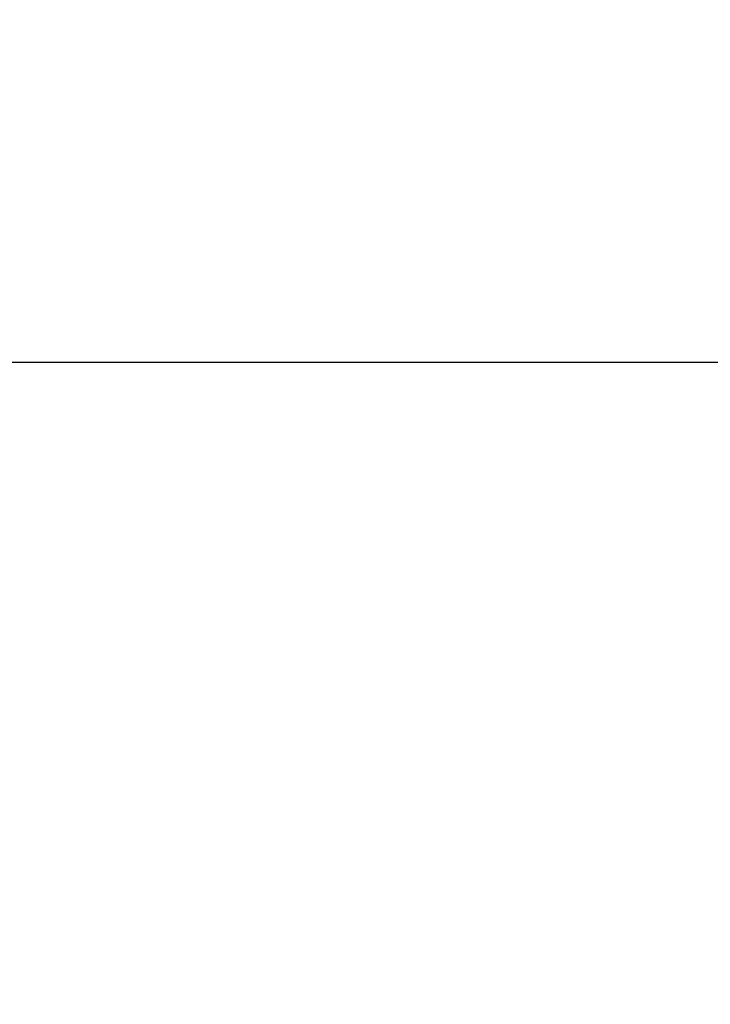
# Model space of a CAD drawing. Units: inches. Extents: x 2337 to 3570, y 1258 to 1938.
# Tile 9 of 30: x 2812 to 2837, y 1642 to 1677. Entities that reach past the tile are written whole.
import ezdxf

# ---------------------------------------------------------------- set-up
doc = ezdxf.new("R2010")
doc.units = ezdxf.units.IN
doc.layers.add('A-ANNO-DIMS', color=2, linetype='Continuous', lineweight=18)
doc.styles.get("Standard").update_dxf_attribs({"font": 'arial.ttf'})
doc.dimstyles.new('ISO-25', dxfattribs={"dimtxt": 9, "dimasz": 2.5, "dimexe": 1.25, "dimexo": 0.625, "dimtad": 1, "dimdec": 1, "dimlunit": 3, "dimtxsty": 'Standard', "dimcen": 2.5, "dimadec": 0, "dimazin": 0, "dimtfac": 1, "dimtdec": 1, "dimtmove": 0, "dimatfit": 3, "dimfxl": 1, "dimarcsym": 0})

# ---------------------------------------------------------------- blocks, each defined once
blk = doc.blocks.new('*D86')
at = {"layer": 'A-ANNO-DIMS', "color": 0, "lineweight": -2, "transparency": 16777216}
for p, q in [((2762.092, 1679.329), (2762.092, 1663.443)), ((2863.836, 1679.329), (2863.836, 1663.443)), ((2762.092, 1664.693), (2617.848, 1664.693)), ((2861.336, 1664.693), (2764.592, 1664.693))]:
    blk.add_line(p, q, dxfattribs=at)
at = {"layer": 'A-ANNO-DIMS', "color": 0, "transparency": 16777216}
for points in [[(2764.592, 1665.109), (2764.592, 1664.276), (2762.092, 1664.693)], [(2861.336, 1665.109), (2861.336, 1664.276), (2863.836, 1664.693)]]:
    blk.add_solid(points, dxfattribs=at)
at = {"layer": 'Defpoints', "color": 0, "transparency": 16777216}
for p in [(2762.092, 1679.954), (2863.836, 1679.954), (2762.092, 1664.693)]:
    blk.add_point(p, dxfattribs=at)
at = {"layer": 'A-ANNO-DIMS', "color": 0, "transparency": 16777216, "insert": (2688.72, 1669.974), "char_height": 9, "attachment_point": 5}
blk.add_mtext('CORNER SOFA 8\'-5 1/2"', dxfattribs=at)

msp = doc.modelspace()

# ---------------------------------------------------------------- dimensions: what is measured, and where the dimension line sits
at = {"layer": 'A-ANNO-DIMS'}
dim = msp.add_linear_dim(base=(2762.092, 1664.693), p1=(2863.836, 1679.954), p2=(2762.092, 1679.954), angle=180, text='CORNER SOFA <>', dimstyle='ISO-25', override={"dimdec": 1, "dimlfac": 1, "dimrnd": 0, "dimzin": 1, "dimdsep": 46, "dimlunit": 4, "dimfrac": 2}, dxfattribs=at)
dim.commit()
dim.dimension.update_dxf_attribs({"geometry": '*D86', "text_midpoint": (2688.72, 1669.974)})

doc.saveas('drawing.dxf')
